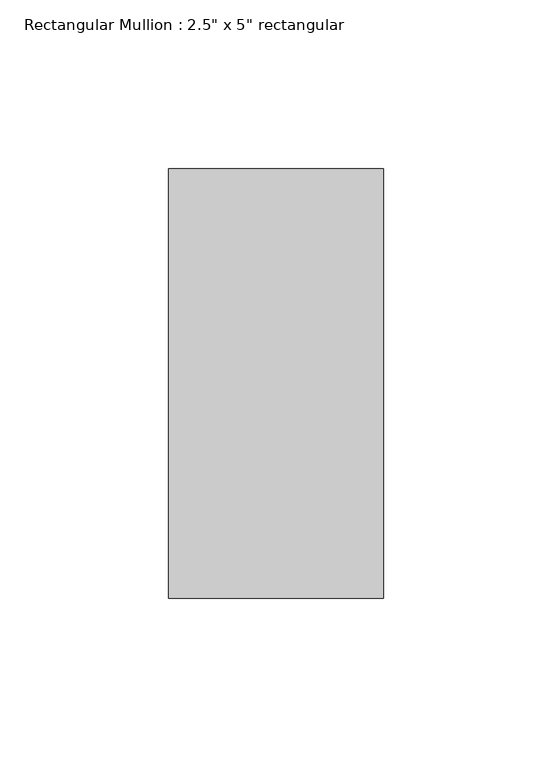
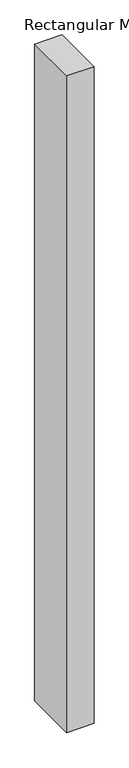
"""IFC4 building model written with IfcOpenShell, lengths in millimetres: member geometry."""

from ifc_helpers import new_model, si_unit, frame, origin, place, context, project, spatial, polyline, outline, extrude, source, transform, mapped, element, save


def member_f53dc333(model_context):
    return source(origin(), model_context, "Body", "SweptSolid", [
        extrude(outline(polyline([(0.0, 63.5), (0.0, -63.5), (-63.5, -63.5), (-63.5, 63.5), (0.0, 63.5)])), frame((0.0, 0.0, -1599.5620987), z_axis=(0.0, 0.0, 1.0), x_axis=(1.0, 0.0, 0.0)), (0.0, 0.0, 1.0), 1599.5620987),
    ])


if __name__ == "__main__":
    model = new_model("IFC4")
    model_context = context("Model", 3, world=origin())
    ifc_project = project(units=[si_unit("LENGTHUNIT", "METRE", prefix="MILLI")], contexts=[model_context])
    site = spatial("IfcSite", under=ifc_project)
    building = spatial("IfcBuilding", under=site)
    placement = place(None, origin())
    member_shape = member_f53dc333(model_context)
    element("IfcMember", 1, ObjectType="Rectangular Mullion : 2.5\" x 5\" rectangular", at=placement, inside=building, context=model_context, shape_type="MappedRepresentation", body=[
        mapped(member_shape, transform((0.0, 0.0, 0.0), x_axis=(1.0, 0.0, 0.0), y_axis=(0.0, 1.0, 0.0), z_axis=(0.0, 0.0, 1.0))),
    ])
    save(model, "model.ifc")

# Revit data of these elements
# Type "Rectangular Mullion : 2.5\" x 5\" rectangular"
#   built-in parameter 1007304 = 0.416667 (stored number, unit not read)
#   built-in parameter 1007301 = 0.104167 (stored number, unit not read)
#   built-in parameter 1007300 = 0.104167 (stored number, unit not read)
# Element 1 (IfcMember, "Rectangular Mullion : 2.5\" x 5\" rectangular")
#   Materials on its faces: "Aluminum"
# Materials
#   "Aluminum": class "Metal", colour RGB 247 247 247, transparency 0, Description = "Aluminum 6061", Cost = 0
